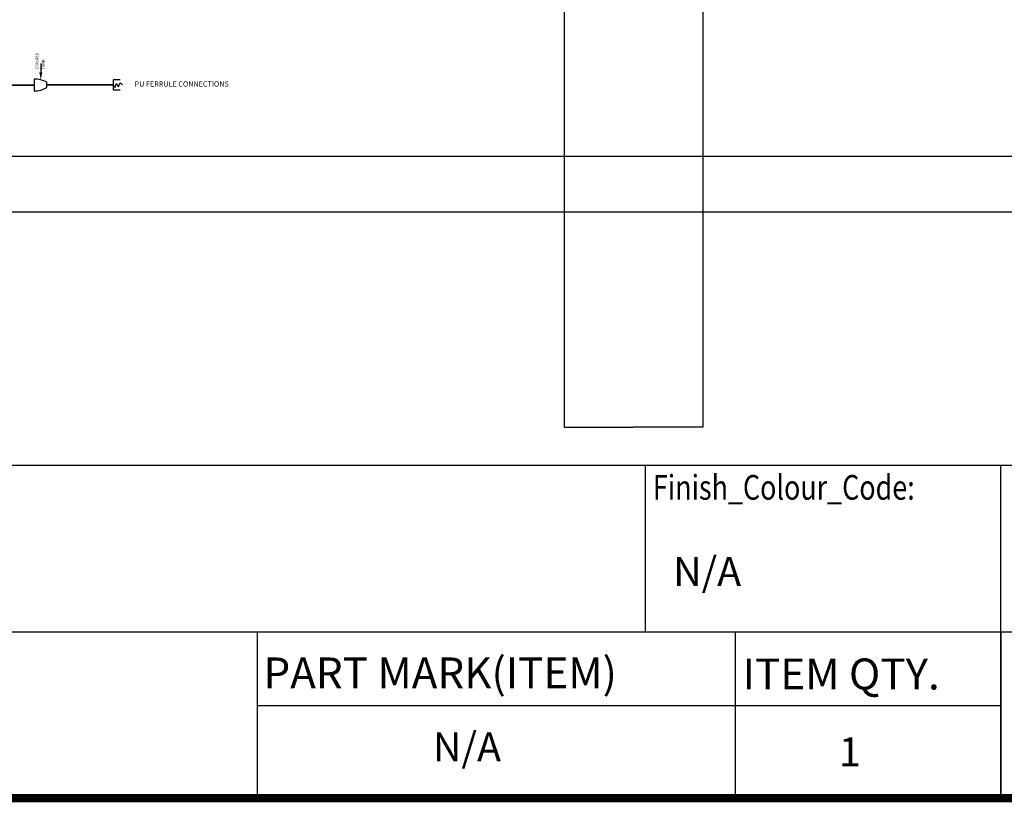
# Model space of a CAD drawing. Units: millimetres. Extents: x 353872 to 441597, y 126154 to 187356.
# Tile 20 of 28: x 399262 to 417572, y 126840 to 141384. Entities that reach past the tile are written whole.
import ezdxf

# ---------------------------------------------------------------- set-up
doc = ezdxf.new("R2010")
doc.units = ezdxf.units.MM
for name, color, linetype, lineweight in [('A-ANNO-DIMS', 2, 'Continuous', 18), ('P-ANNO-TEXT', 7, 'Continuous', 25), ('P-ANNO-TTLB', 7, 'Continuous', 25), ('P-PIPE', 3, 'Continuous', 35), ('P-PIPE-FITT', 6, 'Continuous', 25), ('P-VALV', 2, 'Continuous', 25)]:
    doc.layers.add(name, color=color, linetype=linetype, lineweight=lineweight)
doc.layers.add('AC-UINT', color=2, linetype='Continuous')
doc.styles.add('A1', font='ROMANT.shx', dxfattribs={"height": 200})
doc.styles.add('ROMANC', font='romanc.shx', dxfattribs={"width": 0.75, "height": 4.25})
doc.styles.get("Standard").update_dxf_attribs({"font": 'arial.ttf'})
doc.dimstyles.get("Standard").update_dxf_attribs({"dimtxt": 0.18, "dimasz": 0.18, "dimexe": 0.18, "dimexo": 0.0625, "dimgap": 0.09, "dimtad": 0, "dimtih": 1, "dimtoh": 1, "dimdec": 4, "dimzin": 0, "dimdsep": 46, "dimtxsty": 'Standard', "dimcen": 0.09, "dimadec": 0, "dimazin": 0, "dimtfac": 1, "dimtdec": 4, "dimtofl": 0, "dimtmove": 0, "dimatfit": 3, "dimfxl": 1, "dimtolj": 1, "dimtzin": 0, "dimarcsym": 0})

# ---------------------------------------------------------------- blocks, each defined once
blk = doc.blocks.new('DFSG')
at = {"layer": 'AC-UINT', "ltscale": 3}
blk.add_line((94.324, -27.16), (94.091, -27.16), dxfattribs=at)
blk.add_solid([(94.091, -27.121), (94.091, -27.199), (93.897, -27.16)], dxfattribs=at)
blk = doc.blocks.new('*D27')
at = {"layer": 'A-ANNO-DIMS', "color": 0, "lineweight": -2, "transparency": 16777216}
for p, q in [((366977, 138848), (440591, 138848)), ((440591, 138848), (440591, 138331)), ((440591, 137813), (440591, 138330)), ((366977, 137813), (440591, 137813))]:
    blk.add_line(p, q, dxfattribs=at)
at = {"layer": 'A-ANNO-DIMS', "color": 0, "transparency": 16777216}
for points in [[(440591, 138848), (440591, 138848), (440591, 138848)], [(440591, 137813), (440591, 137813), (440591, 137813)]]:
    blk.add_solid(points, dxfattribs=at)
at = {"layer": 'Defpoints', "color": 0, "transparency": 16777216}
for p in [(366977, 138848), (366977, 137813), (440591, 137813)]:
    blk.add_point(p, dxfattribs=at)
at = {"layer": 'A-ANNO-DIMS', "color": 0, "transparency": 16777216, "insert": (440591, 138330), "char_height": 0.18, "attachment_point": 5}
blk.add_mtext('\\A1;1035.2', dxfattribs=at)
blk = doc.blocks.new('*D31')
at = {"layer": 'A-ANNO-DIMS', "color": 0, "lineweight": -2, "transparency": 16777216}
for p, q in [((409385, 151471), (409385, 133813)), ((411968, 151471), (411968, 133813)), ((409385, 133813), (410676, 133813)), ((411967, 133813), (410677, 133813))]:
    blk.add_line(p, q, dxfattribs=at)
at = {"layer": 'A-ANNO-DIMS', "color": 0, "transparency": 16777216}
for points in [[(409385, 133813), (409385, 133813), (409385, 133813)], [(411967, 133813), (411967, 133813), (411968, 133813)]]:
    blk.add_solid(points, dxfattribs=at)
at = {"layer": 'Defpoints', "color": 0, "transparency": 16777216}
for p in [(409385, 151471), (411968, 151471), (411968, 133813)]:
    blk.add_point(p, dxfattribs=at)
at = {"layer": 'A-ANNO-DIMS', "color": 0, "transparency": 16777216, "insert": (410676, 133813), "char_height": 0.18, "attachment_point": 5}
blk.add_mtext('\\A1;2583', dxfattribs=at)

msp = doc.modelspace()

# ---------------------------------------------------------------- linework, layer by layer
at = {"layer": 'P-ANNO-TTLB'}
for p, q in [((353948.03, 133103.92), (440835.19, 133103.92)), ((410899.77, 130010.13), (410899.77, 133103.92)), ((417504.15, 126916.34), (417504.15, 133103.92)), ((371550.6, 130010.13), (440835.19, 130010.13)), ((403686.43, 130010.13), (417504.15, 130010.13)), ((403686.43, 126916.34), (403686.43, 130010.13)), ((412565.04, 130010.13), (412565.04, 126916.34)), ((417504.15, 130010.13), (417504.15, 126916.34)), ((403686.43, 128641.27), (417504.15, 128641.27))]:
    msp.add_line(p, q, dxfattribs=at)
at = {"layer": 'P-ANNO-TTLB', "const_width": 152.43}
msp.add_lwpolyline([(353948.03, 187280.05), (353948.03, 126916.34), (440835.19, 126916.34), (440835.19, 187280.05)], close=True, dxfattribs=at)
at = {"layer": 'P-PIPE'}
for p, q in [((398670.66, 140169.16), (399531.59, 140169.16)), ((399768.76, 140172.4), (401000.87, 140172.4))]:
    msp.add_line(p, q, dxfattribs=at)
at = {"layer": 'P-VALV'}
for points in [[(399531.59, 140280.43), (399531.59, 140057.89)], [(401128.2, 140263.58), (401000.87, 140263.58), (401000.87, 140081.22), (401128.2, 140081.22)], [(399768.76, 140124.79), (399768.76, 140220.02)]]:
    msp.add_lwpolyline(points, dxfattribs=at)
for centre, radius, start, end in [((399528.49, 139772.52), 507.92, 61.7668, 89.650104), ((399530.12, 140516.96), 459.07, 270.183058, 301.321349)]:
    msp.add_arc(centre, radius, start, end, dxfattribs=at)
msp.add_open_spline([(401000.87, 140172.4), (401014.96, 140147.02), (401047.07, 140089.17), (401050.09, 140256.58), (401106.04, 140085.57), (401118.65, 140237.52), (401156.57, 140191.84), (401173.21, 140171.79)], degree=3, knots=[0, 0, 0, 0, 57.1452101, 130.2277632, 199.75436412, 269.90425966, 324.77408569, 324.77408569, 324.77408569, 324.77408569], dxfattribs=at)

# ---------------------------------------------------------------- block references
at = {"layer": 'P-PIPE-FITT', "xscale": 721.1287546377986, "yscale": 721.1287546377986, "zscale": 721.1287546377986, "rotation": 89.91781771035816}
msp.add_blockref('DFSG', (379971.05, 72581.4), dxfattribs=at)

# ---------------------------------------------------------------- texts
at = {"layer": 'P-ANNO-TEXT'}
for s, p in [('CON.RED', (399610.59, 140459.28)), ('TANK', (399726.56, 140459.28))]:
    msp.add_text(s, height=53.209, rotation=90, dxfattribs=at).set_placement(p)
msp.add_text('PU FERRULE CONNECTIONS', height=98.0901, dxfattribs=at).set_placement((401400.39, 140140.99))
at = {"layer": 'P-ANNO-TTLB', "style": 'A1', "width": 0.8}
msp.add_text('Finish_Colour_Code:', height=458.3394, dxfattribs=at).set_placement((411037.71, 132463.75))
at = {"layer": 'P-ANNO-TTLB'}
for s, height, style, p in [('N/A', 538.476, 'A1', (411412.46, 130859.92)), ('PART MARK(ITEM)', 575.5905, 'ROMANC', (403795.45, 128955.86)), ('ITEM QTY.', 575.591, 'ROMANC', (412706.3, 128936.76)), ('N/A', 539.616, 'ROMANC', (406945.05, 127598.5)), ('1', 539.62, 'ROMANC', (414493.74, 127506.68))]:
    msp.add_text(s, height=height, dxfattribs=dict(at, style=style)).set_placement(p)

# ---------------------------------------------------------------- dimensions: what is measured, and where the dimension line sits
at = {"layer": 'A-ANNO-DIMS'}
dim = msp.add_linear_dim(base=(411967.63, 133812.84), p1=(409384.78, 151470.92), p2=(411967.63, 151470.92), dimstyle='Standard', override={"dimdec": 0, "dimlfac": 1, "dimrnd": 0, "dimzin": 0, "dimdsep": 46, "dimlunit": 2}, dxfattribs=at)
dim.commit()
dim.dimension.update_dxf_attribs({"geometry": '*D31', "text_midpoint": (410676.21, 133812.84)})
dim = msp.add_linear_dim(base=(440591, 137812.84), p1=(366976.76, 138848.06), p2=(366976.76, 137812.84), angle=90, dimstyle='Standard', override={"dimdec": 1, "dimlfac": 1, "dimrnd": 0, "dimzin": 0, "dimdsep": 46, "dimlunit": 2}, dxfattribs=at)
dim.commit()
dim.dimension.update_dxf_attribs({"geometry": '*D27', "text_midpoint": (440591, 138330.45)})

doc.saveas('drawing.dxf')
